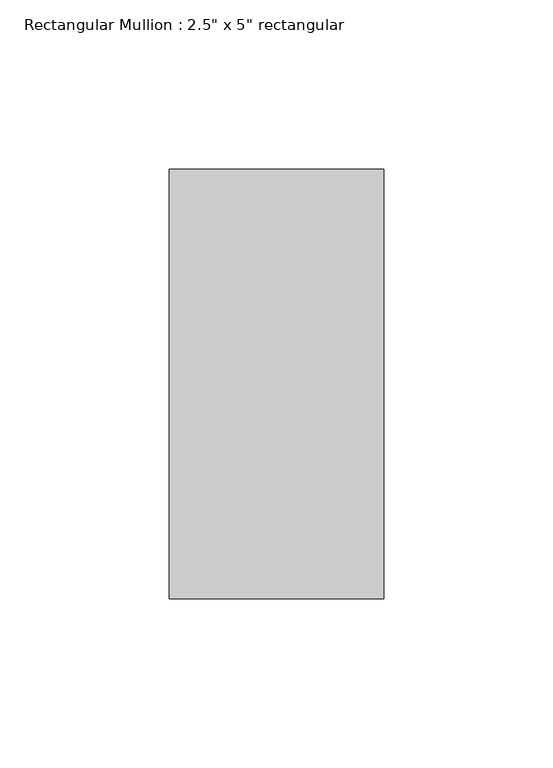
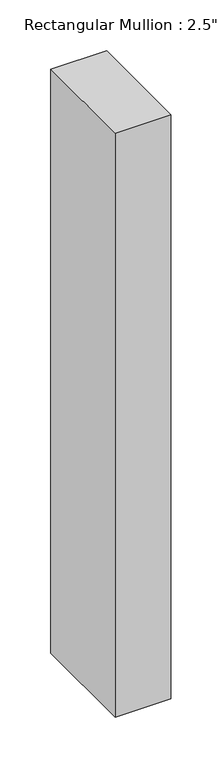
"""IFC4 building model written with IfcOpenShell, lengths in millimetres: member geometry."""

from ifc_helpers import new_model, si_unit, frame, origin, place, context, project, spatial, polyline, outline, extrude, source, transform, mapped, element, save


def member_b3e70a48(model_context):
    return source(origin(), model_context, "Body", "SweptSolid", [
        extrude(outline(polyline([(0.0, 63.5), (0.0, -63.5), (-63.5, -63.5), (-63.5, 63.5), (0.0, 63.5)])), frame((0.0, 0.0, -702.4995873), z_axis=(0.0, 0.0, 1.0), x_axis=(1.0, 0.0, 0.0)), (0.0, 0.0, 1.0), 702.4995873),
    ])


if __name__ == "__main__":
    model = new_model("IFC4")
    model_context = context("Model", 3, world=origin())
    ifc_project = project(units=[si_unit("LENGTHUNIT", "METRE", prefix="MILLI")], contexts=[model_context])
    site = spatial("IfcSite", under=ifc_project)
    building = spatial("IfcBuilding", under=site)
    placement = place(None, origin())
    member_shape = member_b3e70a48(model_context)
    element("IfcMember", 1, ObjectType="Rectangular Mullion : 2.5\" x 5\" rectangular", at=placement, inside=building, context=model_context, shape_type="MappedRepresentation", body=[
        mapped(member_shape, transform((0.0, 0.0, 0.0), x_axis=(1.0, 0.0, 0.0), y_axis=(0.0, 1.0, 0.0), z_axis=(0.0, 0.0, 1.0))),
    ])
    save(model, "model.ifc")

# Revit data of these elements
# Type "Rectangular Mullion : 2.5\" x 5\" rectangular"
#   built-in parameter 1007304 = 0.416667 (stored number, unit not read)
#   built-in parameter 1007301 = 0.104167 (stored number, unit not read)
#   built-in parameter 1007300 = 0.104167 (stored number, unit not read)
# Element 1 (IfcMember, "Rectangular Mullion : 2.5\" x 5\" rectangular")
#   Materials on its faces: "Aluminum"
# Materials
#   "Aluminum": class "Metal", colour RGB 247 247 247, transparency 0, Description = "Aluminum 6061", Cost = 0
